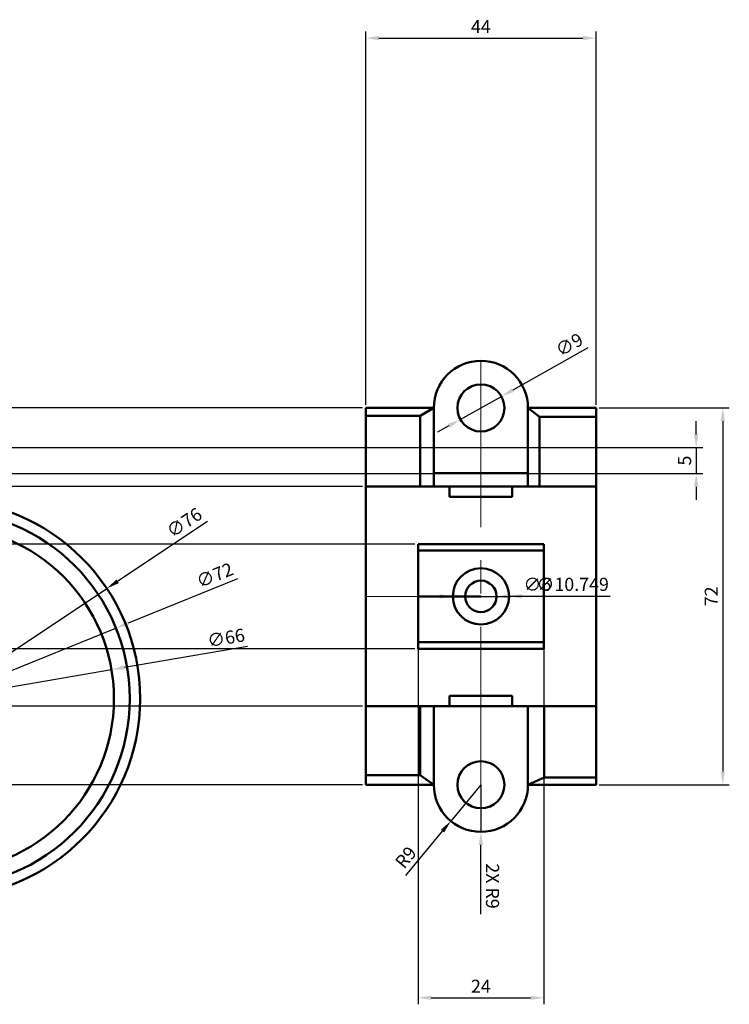
# Model space of a CAD drawing. Units: millimetres. Extents: x 1594 to 1992, y 1694 to 1927.
# Tile 4 of 4: x 1856 to 1992, y 1694 to 1882. Entities that reach past the tile are written whole.
import ezdxf

# ---------------------------------------------------------------- set-up
doc = ezdxf.new("R2010")
doc.units = ezdxf.units.MM
doc.linetypes.add('CENTER', pattern=[50.8, 31.75, -6.35, 6.35, -6.35])
for name, color, linetype, lineweight in [('M-CNTR', 1, 'CENTER', 18), ('M-DIMS', 2, 'Continuous', 25), ('M-OUTL', 7, 'Continuous', 50)]:
    doc.layers.add(name, color=color, linetype=linetype, lineweight=lineweight)
doc.styles.get("Standard").update_dxf_attribs({"font": 'arial.ttf'})
doc.dimstyles.new('ISO-25', dxfattribs={"dimtxt": 2.5, "dimasz": 2.5, "dimexe": 1.25, "dimexo": 0.625, "dimtad": 1, "dimtxsty": 'Standard', "dimcen": 2.5, "dimadec": 0, "dimazin": 0, "dimtfac": 1, "dimtmove": 0, "dimatfit": 3, "dimfxl": 1, "dimarcsym": 0})

# ---------------------------------------------------------------- blocks, each defined once
blk = doc.blocks.new('*D28')
at = {"layer": 'Defpoints', "color": 0, "transparency": 16777216}
for p in [(1872.54, 1773.56), (1809.27, 1731.45)]:
    blk.add_point(p, dxfattribs=at)
at = {"layer": 'M-DIMS', "color": 0, "lineweight": -2, "transparency": 16777216}
for p, q in [((1891.75, 1786.34), (1874.62, 1774.94)), ((1809.27, 1731.45), (1872.54, 1773.56)), ((1807.19, 1730.07), (1805.11, 1728.68))]:
    blk.add_line(p, q, dxfattribs=at)
at = {"layer": 'M-DIMS', "color": 0, "transparency": 16777216}
for points in [[(1874.39, 1775.29), (1874.85, 1774.59), (1872.54, 1773.56)], [(1806.96, 1730.42), (1807.42, 1729.72), (1809.27, 1731.45)]]:
    blk.add_solid(points, dxfattribs=at)
at = {"layer": 'M-DIMS', "color": 0, "transparency": 16777216, "insert": (1887.51, 1785.89), "char_height": 2.5, "attachment_point": 5, "rotation": 33.6408}
blk.add_mtext('∅76', dxfattribs=at)
blk = doc.blocks.new('*D29')
at = {"layer": 'Defpoints', "color": 0, "transparency": 16777216}
for p in [(1874.28, 1766), (1807.53, 1739.01)]:
    blk.add_point(p, dxfattribs=at)
at = {"layer": 'M-DIMS', "color": 0, "lineweight": -2, "transparency": 16777216}
for p, q in [((1897.51, 1775.4), (1876.6, 1766.94)), ((1807.53, 1739.01), (1874.28, 1766)), ((1805.22, 1738.07), (1802.9, 1737.13))]:
    blk.add_line(p, q, dxfattribs=at)
at = {"layer": 'M-DIMS', "color": 0, "transparency": 16777216}
for points in [[(1876.44, 1767.33), (1876.75, 1766.55), (1874.28, 1766)], [(1805.06, 1738.46), (1805.37, 1737.68), (1807.53, 1739.01)]]:
    blk.add_solid(points, dxfattribs=at)
at = {"layer": 'M-DIMS', "color": 0, "transparency": 16777216, "insert": (1893.28, 1775.81), "char_height": 2.5, "attachment_point": 5, "rotation": 22.0218}
blk.add_mtext('∅72', dxfattribs=at)
blk = doc.blocks.new('*D30')
at = {"layer": 'Defpoints', "color": 0, "transparency": 16777216}
for p in [(1873.44, 1758.06), (1808.38, 1746.95)]:
    blk.add_point(p, dxfattribs=at)
at = {"layer": 'M-DIMS', "color": 0, "lineweight": -2, "transparency": 16777216}
for p, q in [((1899.42, 1762.5), (1875.9, 1758.48)), ((1808.38, 1746.95), (1873.44, 1758.06)), ((1805.91, 1746.53), (1803.45, 1746.11))]:
    blk.add_line(p, q, dxfattribs=at)
at = {"layer": 'M-DIMS', "color": 0, "transparency": 16777216}
for points in [[(1875.83, 1758.89), (1875.97, 1758.07), (1873.44, 1758.06)], [(1805.84, 1746.94), (1805.98, 1746.12), (1808.38, 1746.95)]]:
    blk.add_solid(points, dxfattribs=at)
at = {"layer": 'M-DIMS', "color": 0, "transparency": 16777216, "insert": (1895.37, 1763.81), "char_height": 2.5, "attachment_point": 5, "rotation": 9.6936}
blk.add_mtext('∅66', dxfattribs=at)
blk = doc.blocks.new('*D31')
at = {"layer": 'Defpoints', "color": 0, "transparency": 16777216}
for p in [(1947.96, 1810.26), (1940.1, 1805.86)]:
    blk.add_point(p, dxfattribs=at)
at = {"layer": 'M-DIMS', "color": 0, "lineweight": -2, "transparency": 16777216}
for p, q in [((1964.49, 1819.52), (1950.14, 1811.48)), ((1940.1, 1805.86), (1947.96, 1810.26)), ((1937.92, 1804.64), (1935.74, 1803.41))]:
    blk.add_line(p, q, dxfattribs=at)
at = {"layer": 'M-DIMS', "color": 0, "transparency": 16777216}
for points in [[(1949.93, 1811.84), (1950.34, 1811.11), (1947.96, 1810.26)], [(1937.72, 1805), (1938.13, 1804.27), (1940.1, 1805.86)]]:
    blk.add_solid(points, dxfattribs=at)
at = {"layer": 'M-DIMS', "color": 0, "transparency": 16777216, "insert": (1961.08, 1819.87), "char_height": 2.5, "attachment_point": 5, "rotation": 29.2567}
blk.add_mtext('∅9', dxfattribs=at)
blk = doc.blocks.new('*D32')
at = {"layer": 'Defpoints', "color": 0, "transparency": 16777216}
for p in [(1966.03, 1808.06), (1966.03, 1736.06), (1990.26, 1736.06)]:
    blk.add_point(p, dxfattribs=at)
at = {"layer": 'M-DIMS', "color": 0, "lineweight": -2, "transparency": 16777216}
for p, q in [((1966.65, 1808.06), (1991.51, 1808.06)), ((1990.26, 1805.56), (1990.26, 1738.56)), ((1966.65, 1736.06), (1991.51, 1736.06))]:
    blk.add_line(p, q, dxfattribs=at)
at = {"layer": 'M-DIMS', "color": 0, "transparency": 16777216}
for points in [[(1989.84, 1805.56), (1990.67, 1805.56), (1990.26, 1808.06)], [(1989.84, 1738.56), (1990.67, 1738.56), (1990.26, 1736.06)]]:
    blk.add_solid(points, dxfattribs=at)
at = {"layer": 'M-DIMS', "color": 0, "transparency": 16777216, "insert": (1988.38, 1772.06), "char_height": 2.5, "attachment_point": 5, "rotation": 90}
blk.add_mtext('72', dxfattribs=at)
blk = doc.blocks.new('*D33')
at = {"layer": 'Defpoints', "color": 0, "transparency": 16777216}
for p in [(1944.03, 1736.06), (1938.29, 1729.12)]:
    blk.add_point(p, dxfattribs=at)
at = {"layer": 'M-DIMS', "color": 0, "lineweight": -2, "transparency": 16777216}
for p, q in [((1944.03, 1736.06), (1938.29, 1729.12)), ((1929.71, 1718.74), (1936.7, 1727.19))]:
    blk.add_line(p, q, dxfattribs=at)
at = {"layer": 'M-DIMS', "color": 0, "transparency": 16777216}
blk.add_solid([(1936.38, 1727.46), (1937.02, 1726.93), (1938.29, 1729.12)], dxfattribs=at)
at = {"layer": 'M-DIMS', "color": 0, "transparency": 16777216, "insert": (1929.93, 1721.99), "char_height": 2.5, "attachment_point": 5, "rotation": 50.413}
blk.add_mtext('R9', dxfattribs=at)
blk = doc.blocks.new('*D39')
at = {"layer": 'Defpoints', "color": 0, "transparency": 16777216}
for p in [(1840.91, 1800.5), (1840.91, 1795.5), (1985.18, 1795.5)]:
    blk.add_point(p, dxfattribs=at)
at = {"layer": 'M-DIMS', "color": 0, "lineweight": -2, "transparency": 16777216}
for p, q in [((1985.18, 1803), (1985.18, 1805.5)), ((1841.53, 1800.5), (1986.43, 1800.5)), ((1985.18, 1800.5), (1985.18, 1795.5)), ((1841.53, 1795.5), (1986.43, 1795.5)), ((1985.18, 1793), (1985.18, 1790.5))]:
    blk.add_line(p, q, dxfattribs=at)
at = {"layer": 'M-DIMS', "color": 0, "transparency": 16777216}
for points in [[(1984.76, 1803), (1985.6, 1803), (1985.18, 1800.5)], [(1984.76, 1793), (1985.6, 1793), (1985.18, 1795.5)]]:
    blk.add_solid(points, dxfattribs=at)
at = {"layer": 'M-DIMS', "color": 0, "transparency": 16777216, "insert": (1983.28, 1798), "char_height": 2.5, "attachment_point": 5, "rotation": 90}
blk.add_mtext('5', dxfattribs=at)
blk = doc.blocks.new('*D42')
at = {"layer": 'Defpoints', "color": 0, "transparency": 16777216}
for p in [(1966.03, 1878.73), (1922.03, 1808.06), (1966.03, 1808.06)]:
    blk.add_point(p, dxfattribs=at)
at = {"layer": 'M-DIMS', "color": 0, "lineweight": -2, "transparency": 16777216}
for p, q in [((1922.03, 1808.68), (1922.03, 1879.98)), ((1966.03, 1808.68), (1966.03, 1879.98)), ((1924.53, 1878.73), (1963.53, 1878.73))]:
    blk.add_line(p, q, dxfattribs=at)
at = {"layer": 'M-DIMS', "color": 0, "transparency": 16777216}
for points in [[(1924.53, 1879.15), (1924.53, 1878.31), (1922.03, 1878.73)], [(1963.53, 1879.15), (1963.53, 1878.31), (1966.03, 1878.73)]]:
    blk.add_solid(points, dxfattribs=at)
at = {"layer": 'M-DIMS', "color": 0, "transparency": 16777216, "insert": (1944.03, 1880.6), "char_height": 2.5, "attachment_point": 5}
blk.add_mtext('44', dxfattribs=at)
blk = doc.blocks.new('*D43')
at = {"layer": 'Defpoints', "color": 0, "transparency": 16777216}
for p in [(1932.03, 1782.06), (1956.03, 1782.06), (1956.03, 1695.35)]:
    blk.add_point(p, dxfattribs=at)
at = {"layer": 'M-DIMS', "color": 0, "lineweight": -2, "transparency": 16777216}
for p, q in [((1932.03, 1781.43), (1932.03, 1694.1)), ((1956.03, 1781.43), (1956.03, 1694.1)), ((1934.53, 1695.35), (1953.53, 1695.35))]:
    blk.add_line(p, q, dxfattribs=at)
at = {"layer": 'M-DIMS', "color": 0, "transparency": 16777216}
for points in [[(1934.53, 1695.77), (1934.53, 1694.94), (1932.03, 1695.35)], [(1953.53, 1695.77), (1953.53, 1694.94), (1956.03, 1695.35)]]:
    blk.add_solid(points, dxfattribs=at)
at = {"layer": 'M-DIMS', "color": 0, "transparency": 16777216, "insert": (1944.03, 1697.23), "char_height": 2.5, "attachment_point": 5}
blk.add_mtext('24', dxfattribs=at)
blk = doc.blocks.new('*D44')
at = {"layer": 'Defpoints', "color": 0, "transparency": 16777216}
for p in [(1932.03, 1782.06), (1597.57, 1762.06), (1932.03, 1762.06)]:
    blk.add_point(p, dxfattribs=at)
at = {"layer": 'M-DIMS', "color": 0, "lineweight": -2, "transparency": 16777216}
for p, q in [((1931.4, 1782.06), (1596.32, 1782.06)), ((1597.57, 1779.56), (1597.57, 1764.56)), ((1931.4, 1762.06), (1596.32, 1762.06))]:
    blk.add_line(p, q, dxfattribs=at)
at = {"layer": 'M-DIMS', "color": 0, "transparency": 16777216}
for points in [[(1597.15, 1779.56), (1597.99, 1779.56), (1597.57, 1782.06)], [(1597.15, 1764.56), (1597.99, 1764.56), (1597.57, 1762.06)]]:
    blk.add_solid(points, dxfattribs=at)
at = {"layer": 'M-DIMS', "color": 0, "transparency": 16777216, "insert": (1595.67, 1772.06), "char_height": 2.5, "attachment_point": 5, "rotation": 90}
blk.add_mtext('20', dxfattribs=at)
blk = doc.blocks.new('*D45')
at = {"layer": 'Defpoints', "color": 0, "transparency": 16777216}
for p in [(1922.03, 1808.06), (1597.57, 1793.06), (1922.03, 1793.06)]:
    blk.add_point(p, dxfattribs=at)
at = {"layer": 'M-DIMS', "color": 0, "lineweight": -2, "transparency": 16777216}
for p, q in [((1921.4, 1808.06), (1596.32, 1808.06)), ((1597.57, 1805.56), (1597.57, 1795.56)), ((1921.4, 1793.06), (1596.32, 1793.06))]:
    blk.add_line(p, q, dxfattribs=at)
at = {"layer": 'M-DIMS', "color": 0, "transparency": 16777216}
for points in [[(1597.15, 1805.56), (1597.99, 1805.56), (1597.57, 1808.06)], [(1597.15, 1795.56), (1597.99, 1795.56), (1597.57, 1793.06)]]:
    blk.add_solid(points, dxfattribs=at)
at = {"layer": 'M-DIMS', "color": 0, "transparency": 16777216, "insert": (1595.67, 1800.56), "char_height": 2.5, "attachment_point": 5, "rotation": 90}
blk.add_mtext('15', dxfattribs=at)
blk = doc.blocks.new('*D46')
at = {"layer": 'Defpoints', "color": 0, "transparency": 16777216}
for p in [(1922.03, 1751.06), (1597.57, 1736.06), (1922.03, 1736.06)]:
    blk.add_point(p, dxfattribs=at)
at = {"layer": 'M-DIMS', "color": 0, "lineweight": -2, "transparency": 16777216}
for p, q in [((1921.4, 1751.06), (1596.32, 1751.06)), ((1597.57, 1748.56), (1597.57, 1738.56)), ((1921.4, 1736.06), (1596.32, 1736.06))]:
    blk.add_line(p, q, dxfattribs=at)
at = {"layer": 'M-DIMS', "color": 0, "transparency": 16777216}
for points in [[(1597.15, 1748.56), (1597.99, 1748.56), (1597.57, 1751.06)], [(1597.15, 1738.56), (1597.99, 1738.56), (1597.57, 1736.06)]]:
    blk.add_solid(points, dxfattribs=at)
at = {"layer": 'M-DIMS', "color": 0, "transparency": 16777216, "insert": (1595.67, 1743.56), "char_height": 2.5, "attachment_point": 5, "rotation": 90}
blk.add_mtext('15', dxfattribs=at)
blk = doc.blocks.new('*D61')
at = {"layer": 'Defpoints', "color": 0, "transparency": 16777216}
for p in [(1944.03, 1736.06), (1944.03, 1727.06)]:
    blk.add_point(p, dxfattribs=at)
at = {"layer": 'M-DIMS', "color": 0, "lineweight": -2, "transparency": 16777216}
for p, q in [((1944.03, 1736.06), (1944.03, 1727.06)), ((1944.03, 1711.36), (1944.03, 1724.56))]:
    blk.add_line(p, q, dxfattribs=at)
at = {"layer": 'M-DIMS', "color": 0, "transparency": 16777216}
blk.add_solid([(1944.45, 1724.56), (1943.61, 1724.56), (1944.03, 1727.06)], dxfattribs=at)
at = {"layer": 'M-DIMS', "color": 0, "transparency": 16777216, "insert": (1945.93, 1716.71), "char_height": 2.5, "attachment_point": 5, "rotation": 270.0002}
blk.add_mtext('2X R9', dxfattribs=at)
blk = doc.blocks.new('*D62')
at = {"layer": 'Defpoints', "color": 0, "transparency": 16777216}
for p in [(1938.66, 1772.06), (1949.4, 1772.06)]:
    blk.add_point(p, dxfattribs=at)
at = {"layer": 'M-DIMS', "color": 0, "lineweight": -2, "transparency": 16777216}
for p, q in [((1936.16, 1772.06), (1933.66, 1772.06)), ((1938.66, 1772.06), (1949.4, 1772.06)), ((1968.76, 1772.06), (1951.9, 1772.06))]:
    blk.add_line(p, q, dxfattribs=at)
at = {"layer": 'M-DIMS', "color": 0, "transparency": 16777216}
for points in [[(1936.16, 1772.47), (1936.16, 1771.64), (1938.66, 1772.06)], [(1951.9, 1772.47), (1951.9, 1771.64), (1949.4, 1772.06)]]:
    blk.add_solid(points, dxfattribs=at)
at = {"layer": 'M-DIMS', "color": 0, "transparency": 16777216, "insert": (1961.58, 1774.03), "char_height": 2.5, "attachment_point": 5, "rotation": 0.0023}
blk.add_mtext('∅10.749', dxfattribs=at)
blk = doc.blocks.new('*D63')
at = {"layer": 'Defpoints', "color": 0, "transparency": 16777216}
for p in [(1941.03, 1772.06), (1947.03, 1772.06)]:
    blk.add_point(p, dxfattribs=at)
at = {"layer": 'M-DIMS', "color": 0, "lineweight": -2, "transparency": 16777216}
for p, q in [((1938.53, 1772.06), (1936.03, 1772.06)), ((1941.03, 1772.06), (1947.03, 1772.06)), ((1957.64, 1772.06), (1949.53, 1772.06))]:
    blk.add_line(p, q, dxfattribs=at)
at = {"layer": 'M-DIMS', "color": 0, "transparency": 16777216}
for points in [[(1938.53, 1772.47), (1938.53, 1771.64), (1941.03, 1772.06)], [(1949.53, 1772.47), (1949.53, 1771.64), (1947.03, 1772.06)]]:
    blk.add_solid(points, dxfattribs=at)
at = {"layer": 'M-DIMS', "color": 0, "transparency": 16777216, "insert": (1954.83, 1774.03), "char_height": 2.5, "attachment_point": 5, "rotation": 0.0041}
blk.add_mtext('∅6', dxfattribs=at)

msp = doc.modelspace()

# ---------------------------------------------------------------- linework, layer by layer
at = {"layer": 'M-CNTR'}
for p, q in [((1944.03, 1817.0568), (1944.03, 1727.0568)), ((1922.03, 1772.0568), (1966.03, 1772.0568))]:
    msp.add_line(p, q, dxfattribs=at)
at = {"layer": 'M-OUTL'}
for p, q in [((1922.03, 1808.0568), (1922.03, 1736.0568)), ((1935.03, 1808.0568), (1922.03, 1808.0568)), ((1922.03, 1808.0568), (1922.03, 1793.0568)), ((1932.4324, 1806.5819), (1935.03, 1808.0568)), ((1935.03, 1808.0568), (1935.03, 1793.0568)), ((1966.03, 1808.0568), (1953.03, 1808.0568)), ((1953.03, 1808.0568), (1953.03, 1793.0568)), ((1955.2472, 1806.3598), (1953.03, 1808.0568)), ((1966.03, 1736.0568), (1966.03, 1808.0568)), ((1932.4324, 1806.5819), (1922.03, 1806.5819)), ((1932.4324, 1806.5819), (1932.4324, 1793.0568)), ((1955.2472, 1806.3598), (1955.2472, 1793.0568)), ((1966.03, 1806.3598), (1955.2472, 1806.3598)), ((1935.03, 1795.618), (1953.03, 1795.618)), ((1922.03, 1793.0568), (1966.03, 1793.0568)), ((1944.03, 1793.0568), (1938.03, 1793.0568)), ((1938.03, 1793.0568), (1938.03, 1791.0568)), ((1950.03, 1791.0568), (1950.03, 1793.0568)), ((1938.03, 1791.0568), (1950.03, 1791.0568)), ((1932.03, 1772.0568), (1932.03, 1782.0568)), ((1932.03, 1782.0568), (1956.03, 1782.0568)), ((1956.03, 1782.0568), (1956.03, 1762.0568)), ((1932.03, 1780.7982), (1956.03, 1780.7982)), ((1944.03, 1772.0568), (1932.03, 1772.0568)), ((1932.03, 1762.0568), (1932.03, 1772.0568)), ((1956.03, 1763.3015), (1932.03, 1763.3015)), ((1956.03, 1762.0568), (1932.03, 1762.0568)), ((1938.03, 1751.0568), (1938.03, 1753.0568)), ((1938.03, 1753.0568), (1950.03, 1753.0568)), ((1950.03, 1753.0568), (1950.03, 1751.0568)), ((1922.03, 1736.0568), (1922.03, 1751.0568)), ((1922.03, 1751.0568), (1966.03, 1751.0568)), ((1932.4105, 1737.8757), (1932.4105, 1751.0568)), ((1935.03, 1736.0568), (1935.03, 1751.0568)), ((1944.03, 1751.0568), (1938.03, 1751.0568)), ((1953.03, 1736.0568), (1953.03, 1751.0568)), ((1956.1317, 1737.418), (1956.1317, 1751.0568)), ((1922.03, 1737.8757), (1932.4105, 1737.8757)), ((1932.4105, 1737.8757), (1935.03, 1736.0568)), ((1956.1317, 1737.418), (1953.03, 1736.0568)), ((1956.1317, 1737.418), (1966.03, 1737.418)), ((1922.03, 1736.0568), (1935.03, 1736.0568)), ((1953.03, 1736.0568), (1966.03, 1736.0568))]:
    msp.add_line(p, q, dxfattribs=at)
for centre, radius in [((1944.03, 1808.0568), 4.5), ((1840.9068, 1752.5048), 38), ((1840.9068, 1752.5048), 36), ((1840.9068, 1752.5048), 33), ((1944.03, 1772.0568), 5.3744), ((1944.03, 1772.0568), 3), ((1944.03, 1736.0568), 4.5)]:
    msp.add_circle(centre, radius, dxfattribs=at)
for centre, start, end in [((1944.03, 1808.0568), 0, 180), ((1944.03, 1736.0568), 180, 0)]:
    msp.add_arc(centre, 9, start, end, dxfattribs=at)

# ---------------------------------------------------------------- dimensions: what is measured, and where the dimension line sits
at = {"layer": 'M-DIMS'}
for base, p1, p2, picture, middle in [((1966.03, 1878.7297), (1922.03, 1808.0568), (1966.03, 1808.0568), '*D42', (1944.03, 1880.6047)), ((1956.03, 1695.3548), (1932.03, 1782.0568), (1956.03, 1782.0568), '*D43', (1944.03, 1697.2349))]:
    dim = msp.add_linear_dim(base=base, p1=p1, p2=p2, dimstyle='ISO-25', override={"dimdec": 0, "dimlfac": 1, "dimrnd": 0, "dimzin": 0, "dimdsep": 46, "dimlunit": 2}, dxfattribs=at)
    dim.commit()
    dim.dimension.update_dxf_attribs({"geometry": picture, "text_midpoint": middle})
for p1, p2, override, picture, middle in [((1940.104, 1805.8575), (1947.9559, 1810.256), {"dimclrd": 0, "dimclre": 0, "dimclrt": 0}, '*D31', (1962.0455, 1818.1487)), ((1809.2708, 1731.4534), (1872.5428, 1773.5562), {"dimclrd": 0, "dimclre": 0, "dimclrt": 0}, '*D28', (1888.6064, 1784.2453)), ((1807.5334, 1739.0062), (1874.2803, 1766.0034), {"dimclrd": 0, "dimclre": 0, "dimclrt": 0}, '*D29', (1894.0198, 1773.9874)), ((1938.6556, 1772.0566), (1949.4043, 1772.057), {"dimdec": 3, "dimlfac": 1, "dimrnd": 0, "dimzin": 0, "dimdsep": 46, "dimlunit": 2}, '*D62', (1961.5812, 1772.0575)), ((1808.378, 1746.9483), (1873.4357, 1758.0613), {"dimclrd": 0, "dimclre": 0, "dimclrt": 0}, '*D30', (1895.6999, 1761.8644))]:
    dim = msp.add_diameter_dim_2p(p1=p1, p2=p2, dimstyle='ISO-25', override=override, dxfattribs=at)
    dim.commit()
    dim.dimension.update_dxf_attribs({"geometry": picture, "text_midpoint": middle, "dimtype": 163})
for base, p1, p2, override, picture, middle in [((1597.571, 1793.0568), (1922.03, 1808.0568), (1922.03, 1793.0568), {"dimdec": 0, "dimlfac": 1, "dimrnd": 0, "dimzin": 0, "dimdsep": 46, "dimlunit": 2}, '*D45', (1595.6695, 1800.5568)), ((1990.2575, 1736.0568), (1966.03, 1808.0568), (1966.03, 1736.0568), {"dimclrd": 0, "dimclre": 0, "dimclrt": 0}, '*D32', (1988.3774, 1772.0568)), ((1985.18, 1795.5048), (1840.9068, 1800.5048), (1840.9068, 1795.5048), {"dimdec": 0, "dimlfac": 1, "dimrnd": 0, "dimzin": 0, "dimdsep": 46, "dimlunit": 2}, '*D39', (1983.2836, 1798.0048)), ((1597.571, 1762.0568), (1932.03, 1782.0568), (1932.03, 1762.0568), {"dimdec": 0, "dimlfac": 1, "dimrnd": 0, "dimzin": 0, "dimdsep": 46, "dimlunit": 2}, '*D44', (1595.6695, 1772.0568)), ((1597.571, 1736.0568), (1922.03, 1751.0568), (1922.03, 1736.0568), {"dimdec": 0, "dimlfac": 1, "dimrnd": 0, "dimzin": 0, "dimdsep": 46, "dimlunit": 2}, '*D46', (1595.6695, 1743.5568))]:
    dim = msp.add_linear_dim(base=base, p1=p1, p2=p2, angle=90, dimstyle='ISO-25', override=override, dxfattribs=at)
    dim.commit()
    dim.dimension.update_dxf_attribs({"geometry": picture, "text_midpoint": middle})
dim = msp.add_diameter_dim_2p(p1=(1941.03, 1772.0566), p2=(1947.03, 1772.057), dimstyle='ISO-25', override={"dimdec": 0, "dimlfac": 1, "dimrnd": 0, "dimzin": 0, "dimdsep": 46, "dimlunit": 2}, dxfattribs=at)
dim.commit()
dim.dimension.update_dxf_attribs({"geometry": '*D63', "text_midpoint": (1954.8335, 1772.0576)})
dim = msp.add_radius_dim(center=(1944.03, 1736.0568), mpoint=(1938.2947, 1729.1209), dimstyle='ISO-25', override={"dimclrd": 0, "dimclre": 0, "dimclrt": 0}, dxfattribs=at)
dim.commit()
dim.dimension.update_dxf_attribs({"geometry": '*D33', "text_midpoint": (1931.3993, 1720.7819), "dimtype": 164})
dim = msp.add_radius_dim(center=(1944.03, 1736.0568), mpoint=(1944.03, 1727.0568), text='2X <>', dimstyle='ISO-25', override={"dimdec": 0, "dimlfac": 1, "dimrnd": 0, "dimzin": 0, "dimdsep": 46, "dimlunit": 2}, dxfattribs=at)
dim.commit()
dim.dimension.update_dxf_attribs({"geometry": '*D61', "text_midpoint": (1945.9315, 1716.7064)})

doc.saveas('drawing.dxf')
